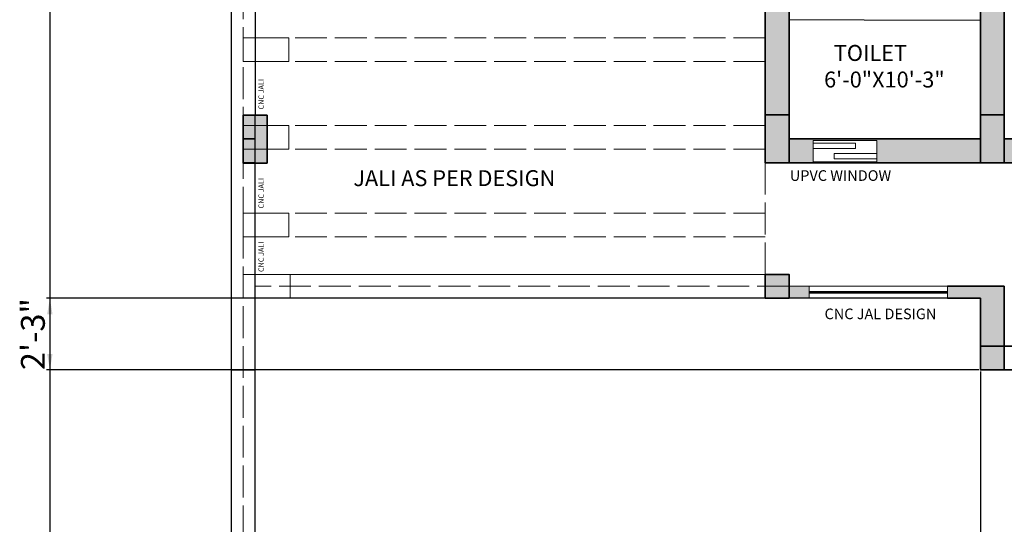
# Model space of a CAD drawing. Units: millimetres. Extents: x 595116 to 630915, y 909473 to 920225.
# Tile 128 of 134: x 630214 to 630585, y 919276 to 919466. Entities that reach past the tile are written whole.
import ezdxf

# ---------------------------------------------------------------- set-up
doc = ezdxf.new("R2010")
doc.units = ezdxf.units.MM
doc.linetypes.add('ACAD_ISO02W100', pattern=[15, 12, -3])
for name, color, linetype, lineweight in [('A-AREA-IDEN', 7, 'Continuous', 20), ('A-FLOR-FIXT', 9, 'Continuous', 18), ('A-FLOR-SCRN', 31, 'Continuous', 18), ('A-FLOR-SCRN-OVHD', 31, 'ACAD_ISO02W100', 13), ('A-WALL', 1, 'Continuous', 35), ('A-WALL-PATT', 8, 'Continuous', 13), ('C-PROP', 7, 'Continuous', 25), ('C-PROP-REF', 240, 'ACAD_ISO02W100', 13), ('Column', 6, 'Continuous', 35), ('Dimension', 3, 'Continuous', 18), ('Text', 7, 'Continuous', 18), ('Windows', 33, 'Continuous', 18)]:
    doc.layers.add(name, color=color, linetype=linetype, lineweight=lineweight)
doc.styles.get("Standard").update_dxf_attribs({"font": 'arial.ttf'})
doc.dimstyles.new('ISO-25', dxfattribs={"dimtxt": 9, "dimasz": 6, "dimexe": 1.25, "dimexo": 0.625, "dimtad": 1, "dimlunit": 4, "dimtxsty": 'Standard', "dimcen": 2.5, "dimadec": 0, "dimazin": 0, "dimtfac": 1, "dimtmove": 0, "dimatfit": 3, "dimfxl": 1, "dimarcsym": 0})

# ---------------------------------------------------------------- blocks, each defined once
blk = doc.blocks.new('COLUMN-SQUARE-9IN')
h = blk.add_hatch(color=256)
h.dxf.hatch_style = 1
h.paths.add_polyline_path([(9, 9), (0, 9), (0, 0), (9, 0)])
blk.add_lwpolyline([(0, 9), (9, 9), (9, 0), (0, 0)], close=True)
blk = doc.blocks.new('COLUMN-RECT-9X18')
h = blk.add_hatch(color=256)
h.dxf.hatch_style = 1
h.paths.add_polyline_path([(9, 18), (0, 18), (0, 0), (9, 0)])
blk.add_lwpolyline([(0, 18), (9, 18), (9, 0), (0, 0)], close=True)
blk = doc.blocks.new('*D214')
at = {"layer": 'Defpoints', "color": 0, "transparency": 16777216}
for p in [(630293.6, 920089.43), (630225.3, 919146.43), (630293.6, 919146.43)]:
    blk.add_point(p, dxfattribs=at)
at = {"layer": 'Dimension', "color": 0, "lineweight": -2, "transparency": 16777216}
for p, q in [((630292.97, 920089.43), (630224.05, 920089.43)), ((630225.3, 920083.43), (630225.3, 919152.43)), ((630292.97, 919146.43), (630224.05, 919146.43))]:
    blk.add_line(p, q, dxfattribs=at)
at = {"layer": 'Dimension', "color": 0, "transparency": 16777216}
for points in [[(630224.3, 920083.43), (630226.3, 920083.43), (630225.3, 920089.43)], [(630224.3, 919152.43), (630226.3, 919152.43), (630225.3, 919146.43)]]:
    blk.add_solid(points, dxfattribs=at)
at = {"layer": 'Dimension', "color": 0, "transparency": 16777216, "insert": (630220.08, 919617.93), "char_height": 9, "attachment_point": 5, "rotation": 90}
blk.add_mtext('78\'-7"', dxfattribs=at)
blk = doc.blocks.new('*D218')
at = {"layer": 'Defpoints', "color": 0, "transparency": 16777216}
for p in [(630575.6, 919333.93), (630742.1, 919333.93), (630742.1, 919078.13)]:
    blk.add_point(p, dxfattribs=at)
at = {"layer": 'Dimension', "color": 0, "lineweight": -2, "transparency": 16777216}
for p, q in [((630575.6, 919333.3), (630575.6, 919076.88)), ((630742.1, 919333.3), (630742.1, 919076.88)), ((630581.6, 919078.13), (630736.1, 919078.13))]:
    blk.add_line(p, q, dxfattribs=at)
at = {"layer": 'Dimension', "color": 0, "transparency": 16777216}
for points in [[(630581.6, 919079.13), (630581.6, 919077.13), (630575.6, 919078.13)], [(630736.1, 919079.13), (630736.1, 919077.13), (630742.1, 919078.13)]]:
    blk.add_solid(points, dxfattribs=at)
at = {"layer": 'Dimension', "color": 0, "transparency": 16777216, "insert": (630658.85, 919083.41), "char_height": 9, "attachment_point": 5}
blk.add_mtext('13\'-10 1/2"', dxfattribs=at)
blk = doc.blocks.new('*D219')
at = {"layer": 'Defpoints', "color": 0, "transparency": 16777216}
for p in [(630575.6, 919360.93), (630225.3, 919333.93), (630575.6, 919333.93)]:
    blk.add_point(p, dxfattribs=at)
at = {"layer": 'Dimension', "color": 0, "lineweight": -2, "transparency": 16777216}
for p, q in [((630574.97, 919360.93), (630224.05, 919360.93)), ((630225.3, 919354.93), (630225.3, 919339.93)), ((630574.97, 919333.93), (630224.05, 919333.93))]:
    blk.add_line(p, q, dxfattribs=at)
at = {"layer": 'Dimension', "color": 0, "transparency": 16777216}
for points in [[(630224.3, 919354.93), (630226.3, 919354.93), (630225.3, 919360.93)], [(630224.3, 919339.93), (630226.3, 919339.93), (630225.3, 919333.93)]]:
    blk.add_solid(points, dxfattribs=at)
at = {"layer": 'Dimension', "color": 0, "transparency": 16777216, "insert": (630220.07, 919347.43), "char_height": 9, "attachment_point": 5, "rotation": 90}
blk.add_mtext('2\'-3"', dxfattribs=at)

msp = doc.modelspace()

# ---------------------------------------------------------------- hatches: boundary and pattern name
at = {"layer": 'A-WALL-PATT'}
h = msp.add_hatch(color=256, dxfattribs=at)
h.dxf.hatch_style = 1
h.paths.add_polyline_path([(630503.596, 919609.928), (630496.096, 919609.928), (630496.096, 919591.928), (630494.596, 919591.928), (630494.596, 919429.828), (630496.096, 919429.828), (630496.096, 919411.928), (630512.596, 919411.928), (630512.596, 919420.323), (630536.596, 919420.323), (630536.596, 919411.928), (630575.596, 919411.928), (630575.596, 919420.928), (630503.596, 919420.928)])
h = msp.add_hatch(color=256, dxfattribs=at)
h.dxf.hatch_style = 1
h.paths.add_polyline_path([(630584.596, 919609.928), (630577.096, 919609.928), (630577.096, 919591.928), (630575.596, 919591.928), (630575.596, 919552.928), (630533.596, 919552.928), (630533.596, 919548.428), (630575.596, 919548.428), (630575.596, 919429.928), (630577.096, 919429.928), (630577.096, 919411.928), (630608.596, 919411.928), (630608.596, 919420.928), (630584.596, 919420.928)])
h = msp.add_hatch(color=256, dxfattribs=at)
h.dxf.hatch_style = 1
h.paths.add_polyline_path([(630511.093, 919365.428), (630503.596, 919365.428), (630503.596, 919360.928), (630511.093, 919360.928)])
h = msp.add_hatch(color=256, dxfattribs=at)
h.dxf.hatch_style = 1
h.paths.add_polyline_path([(630584.596, 919365.428), (630563.266, 919365.428), (630563.266, 919360.928), (630575.596, 919360.928), (630575.596, 919342.928), (630584.596, 919342.928)])

# ---------------------------------------------------------------- linework, layer by layer
at = {"layer": 'A-FLOR-FIXT'}
for p, q in [((630531.887, 919465.77), (630503.596, 919465.77)), ((630575.596, 919465.669), (630531.887, 919465.669))]:
    msp.add_line(p, q, dxfattribs=at)
at = {"layer": 'A-FLOR-SCRN'}
for p, q in [((630494.596, 919369.928), (630302.596, 919369.928)), ((630511.093, 919365.428), (630503.596, 919365.428)), ((630503.596, 919365.428), (630503.596, 919360.928)), ((630511.093, 919365.428), (630511.093, 919360.928)), ((630563.266, 919365.428), (630511.093, 919365.428)), ((630563.266, 919365.428), (630563.266, 919360.928)), ((630494.596, 919360.928), (630302.596, 919360.928)), ((630511.093, 919360.928), (630494.596, 919360.928)), ((630511.093, 919363.527), (630563.266, 919363.527)), ((630511.093, 919363.178), (630563.266, 919363.178)), ((630511.093, 919362.785), (630563.266, 919362.785)), ((630563.266, 919360.928), (630511.093, 919360.928))]:
    msp.add_line(p, q, dxfattribs=at)
for points in [[(630298.096, 919459.015), (630315.223, 919459.015), (630315.223, 919450.015), (630298.096, 919450.015)], [(630298.096, 919426.015), (630315.223, 919426.015), (630315.223, 919417.015), (630298.096, 919417.015)], [(630298.096, 919393.015), (630315.223, 919393.015), (630315.223, 919384.015), (630298.096, 919384.015)], [(630298.096, 919369.928), (630315.771, 919369.928), (630315.771, 919360.928), (630298.096, 919360.928)]]:
    msp.add_lwpolyline(points, close=True, dxfattribs=at)
at = {"layer": 'A-FLOR-SCRN-OVHD'}
for p, q in [((630302.596, 919459.015), (630494.596, 919459.015)), ((630302.596, 919450.015), (630494.596, 919450.015)), ((630302.596, 919426.015), (630494.596, 919426.015)), ((630302.596, 919417.015), (630494.596, 919417.015)), ((630494.596, 919411.928), (630494.596, 919369.928)), ((630302.596, 919393.015), (630494.596, 919393.015)), ((630302.596, 919384.015), (630494.596, 919384.015)), ((630503.596, 919365.428), (630302.596, 919365.428))]:
    msp.add_line(p, q, dxfattribs=at)
at = {"layer": 'A-WALL'}
for p, q in [((630494.596, 919411.928), (630494.596, 919609.928)), ((630503.596, 919420.928), (630503.596, 919609.928)), ((630584.596, 919420.928), (630584.596, 919609.928)), ((630575.596, 919420.928), (630575.596, 919548.428)), ((630298.096, 919420.928), (630302.596, 919420.928)), ((630503.596, 919420.928), (630575.596, 919420.928)), ((630584.596, 919420.928), (630737.596, 919420.928)), ((630298.096, 919411.928), (630302.596, 919411.928)), ((630494.596, 919411.928), (630733.096, 919411.928)), ((630494.596, 919365.428), (630494.596, 919360.928)), ((630503.596, 919365.428), (630503.596, 919360.928)), ((630584.596, 919365.428), (630563.266, 919365.428)), ((630584.596, 919365.428), (630584.596, 919342.928)), ((630575.596, 919360.928), (630563.266, 919360.928)), ((630575.596, 919360.928), (630575.596, 919333.928)), ((630584.596, 919342.928), (630733.096, 919342.928)), ((630302.596, 919333.928), (630293.596, 919333.928)), ((630575.596, 919333.928), (630742.096, 919333.928))]:
    msp.add_line(p, q, dxfattribs=at)
at = {"layer": 'C-PROP'}
for p, q in [((630293.596, 919516.015), (630293.596, 919146.428)), ((630302.596, 919516.015), (630302.596, 919429.828)), ((630302.596, 919155.428), (630302.596, 919429.828))]:
    msp.add_line(p, q, dxfattribs=at)
at = {"layer": 'C-PROP-REF'}
msp.add_line((630298.096, 919150.928), (630298.096, 920084.928), dxfattribs=at)
at = {"layer": 'Windows'}
for p, q in [((630512.596, 919420.928), (630536.596, 919420.928)), ((630512.596, 919420.323), (630512.596, 919411.928)), ((630536.596, 919420.323), (630536.596, 919411.928)), ((630512.596, 919419.357), (630528.596, 919419.357)), ((630512.596, 919411.928), (630536.596, 919411.928))]:
    msp.add_line(p, q, dxfattribs=at)
msp.add_lwpolyline([(630512.596, 919420.323), (630536.596, 919420.323), (630536.596, 919412.338), (630512.596, 919412.338)], close=True, dxfattribs=at)
for points in [[(630512.596, 919417.357), (630528.596, 919417.357), (630528.596, 919419.357)], [(630536.596, 919413.357), (630520.596, 919413.357), (630520.596, 919415.357), (630536.596, 919415.357)]]:
    msp.add_lwpolyline(points, dxfattribs=at)

# ---------------------------------------------------------------- block references
at = {"layer": 'Column'}
for name, p in [('COLUMN-RECT-9X18', (630298.096, 919411.828)), ('COLUMN-RECT-9X18', (630494.596, 919411.928)), ('COLUMN-RECT-9X18', (630575.596, 919411.928)), ('COLUMN-SQUARE-9IN', (630494.596, 919360.928)), ('COLUMN-SQUARE-9IN', (630575.596, 919333.928))]:
    msp.add_blockref(name, p, dxfattribs=at)

# ---------------------------------------------------------------- texts
at = {"layer": 'A-AREA-IDEN', "insert": (630509.414, 919456.265), "char_height": 6, "attachment_point": 1}
msp.add_mtext_dynamic_manual_height_columns('{      TOILET\\P    6\'-0"X10\'-3"}', width=83.57324, gutter_width=12.5, heights=[0], dxfattribs=at)
at = {"layer": 'Text', "char_height": 2, "attachment_point": 1, "rotation": 90}
for insert in [(630303.831, 919431.988), (630303.831, 919394.722), (630303.831, 919370.812)]:
    msp.add_mtext_dynamic_manual_height_columns('{CNC JALI}', width=125.26422, gutter_width=12.5, heights=[0], dxfattribs=dict(at, insert=insert))
at = {"layer": 'Text', "attachment_point": 1}
for s, width, insert, char_height in [('{JALI AS PER DESIGN}', 125.26422, (630339.535, 919409.133), 6), ('{ UPVC WINDOW}', 61.33456, (630502.631, 919409.113), 4), ('{CNC JAL DESIGN}', 125.26422, (630516.926, 919357.042), 4)]:
    msp.add_mtext_dynamic_manual_height_columns(s, width=width, gutter_width=12.5, heights=[0], dxfattribs=dict(at, insert=insert, char_height=char_height))

# ---------------------------------------------------------------- dimensions: what is measured, and where the dimension line sits
at = {"layer": 'Dimension'}
for base, p1, p2, picture, middle in [((630225.296, 919146.428), (630293.596, 920089.428), (630293.596, 919146.428), '*D214', (630220.076, 919617.928)), ((630225.296, 919333.928), (630575.596, 919360.928), (630575.596, 919333.928), '*D219', (630220.073, 919347.428))]:
    dim = msp.add_linear_dim(base=base, p1=p1, p2=p2, angle=90, dimstyle='ISO-25', override={"dimdec": 1, "dimlfac": 1, "dimrnd": 0, "dimzin": 1, "dimdsep": 46, "dimlunit": 4, "dimfrac": 2}, dxfattribs=at)
    dim.commit()
    dim.dimension.update_dxf_attribs({"geometry": picture, "text_midpoint": middle})
dim = msp.add_linear_dim(base=(630742.096, 919078.128), p1=(630575.596, 919333.928), p2=(630742.096, 919333.928), dimstyle='ISO-25', override={"dimdec": 1, "dimlfac": 1, "dimrnd": 0, "dimzin": 1, "dimdsep": 46, "dimlunit": 4, "dimfrac": 2}, dxfattribs=at)
dim.commit()
dim.dimension.update_dxf_attribs({"geometry": '*D218', "text_midpoint": (630658.846, 919083.409)})

doc.saveas('drawing.dxf')
